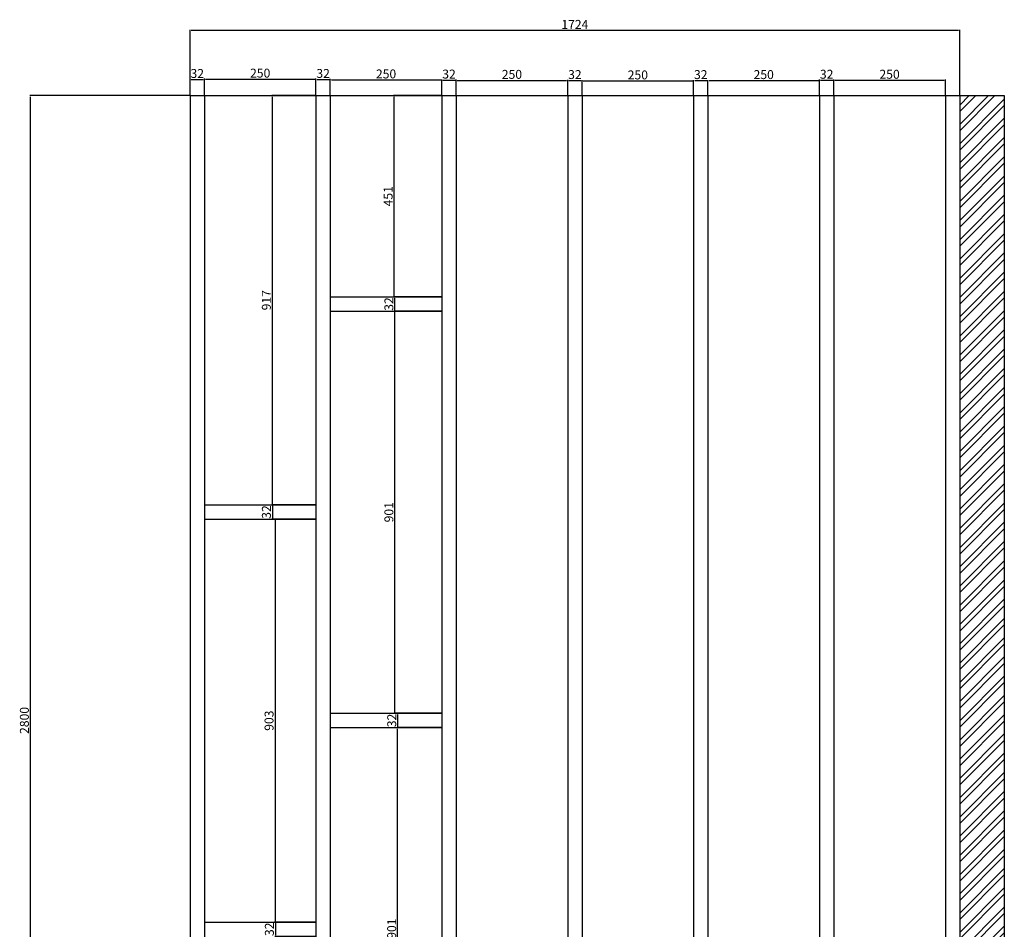
# Model space of a CAD drawing. Units: millimetres. Extents: x 1898 to 8115, y 727 to 4291.
# Tile 2 of 7: x 1898 to 4104, y 2252 to 4291. Entities that reach past the tile are written whole.
import ezdxf

# ---------------------------------------------------------------- set-up
doc = ezdxf.new("R2010")
doc.units = ezdxf.units.MM
for name, color, linetype, lineweight in [('A-ANNO-DIMS', 2, 'Continuous', 18), ('A-DETL', 7, 'Continuous', 25), ('A-DETL-PATT', 8, 'Continuous', 13)]:
    doc.layers.add(name, color=color, linetype=linetype, lineweight=lineweight)
doc.styles.get("Standard").update_dxf_attribs({"font": 'arial.ttf'})
doc.dimstyles.new('ISO-25', dxfattribs={"dimtxt": 20, "dimasz": 2.5, "dimexe": 1.25, "dimexo": 0.625, "dimtad": 1, "dimtxsty": 'Standard', "dimcen": 2.5, "dimadec": 0, "dimazin": 0, "dimtfac": 1, "dimtmove": 0, "dimatfit": 3, "dimfxl": 1, "dimarcsym": 0})

# ---------------------------------------------------------------- blocks, each defined once
blk = doc.blocks.new('*D16')
at = {"layer": 'A-ANNO-DIMS', "color": 0, "lineweight": -2, "transparency": 16777216}
for p, q in [((2279.1, 4120.5), (1920.7, 4120.5)), ((1921.9, 1323), (1921.9, 4118)), ((2279.1, 1320.5), (1920.7, 1320.5))]:
    blk.add_line(p, q, dxfattribs=at)
at = {"layer": 'A-ANNO-DIMS', "color": 0, "transparency": 16777216}
for points in [[(1921.5, 4118), (1922.3, 4118), (1921.9, 4120.5)], [(1921.5, 1323), (1922.3, 1323), (1921.9, 1320.5)]]:
    blk.add_solid(points, dxfattribs=at)
at = {"layer": 'Defpoints', "color": 0, "transparency": 16777216}
for p in [(1921.9, 4120.5), (2279.7, 4120.5), (2279.7, 1320.5)]:
    blk.add_point(p, dxfattribs=at)
at = {"layer": 'A-ANNO-DIMS', "color": 0, "transparency": 16777216, "insert": (1911.1, 2720.5), "char_height": 20, "attachment_point": 5, "rotation": 90}
blk.add_mtext('2800', dxfattribs=at)
blk = doc.blocks.new('*D17')
at = {"layer": 'A-ANNO-DIMS', "color": 0, "lineweight": -2, "transparency": 16777216}
for p, q in [((2279.7, 4121.1), (2279.7, 4268.1)), ((2282.2, 4266.9), (4001.2, 4266.9)), ((4003.7, 4121.1), (4003.7, 4268.1))]:
    blk.add_line(p, q, dxfattribs=at)
at = {"layer": 'A-ANNO-DIMS', "color": 0, "transparency": 16777216}
for points in [[(2282.2, 4267.3), (2282.2, 4266.4), (2279.7, 4266.9)], [(4001.2, 4267.3), (4001.2, 4266.4), (4003.7, 4266.9)]]:
    blk.add_solid(points, dxfattribs=at)
at = {"layer": 'Defpoints', "color": 0, "transparency": 16777216}
for p in [(4003.7, 4266.9), (2279.7, 4120.5), (4003.7, 4120.5)]:
    blk.add_point(p, dxfattribs=at)
at = {"layer": 'A-ANNO-DIMS', "color": 0, "transparency": 16777216, "insert": (3141.7, 4277.5), "char_height": 20, "attachment_point": 5}
blk.add_mtext('1724', dxfattribs=at)
blk = doc.blocks.new('*D18')
at = {"layer": 'A-ANNO-DIMS', "color": 0, "lineweight": -2, "transparency": 16777216}
for p, q in [((2279.7, 4121.1), (2279.7, 4158)), ((2282.2, 4156.8), (2309.2, 4156.8)), ((2311.7, 4121.1), (2311.7, 4158))]:
    blk.add_line(p, q, dxfattribs=at)
at = {"layer": 'A-ANNO-DIMS', "color": 0, "transparency": 16777216}
for points in [[(2282.2, 4157.2), (2282.2, 4156.4), (2279.7, 4156.8)], [(2309.2, 4157.2), (2309.2, 4156.4), (2311.7, 4156.8)]]:
    blk.add_solid(points, dxfattribs=at)
at = {"layer": 'Defpoints', "color": 0, "transparency": 16777216}
for p in [(2311.7, 4156.8), (2279.7, 4120.5), (2311.7, 4120.5)]:
    blk.add_point(p, dxfattribs=at)
at = {"layer": 'A-ANNO-DIMS', "color": 0, "transparency": 16777216, "insert": (2295.7, 4167.6), "char_height": 20, "attachment_point": 5}
blk.add_mtext('32', dxfattribs=at)
blk = doc.blocks.new('*D19')
at = {"layer": 'A-ANNO-DIMS', "color": 0, "lineweight": -2, "transparency": 16777216}
for p, q in [((2311.7, 4121.1), (2311.7, 4158.7)), ((2314.2, 4157.5), (2559.2, 4157.5)), ((2561.7, 4121.1), (2561.7, 4158.7))]:
    blk.add_line(p, q, dxfattribs=at)
at = {"layer": 'A-ANNO-DIMS', "color": 0, "transparency": 16777216}
for points in [[(2314.2, 4157.9), (2314.2, 4157), (2311.7, 4157.5)], [(2559.2, 4157.9), (2559.2, 4157), (2561.7, 4157.5)]]:
    blk.add_solid(points, dxfattribs=at)
at = {"layer": 'Defpoints', "color": 0, "transparency": 16777216}
for p in [(2561.7, 4157.5), (2311.7, 4120.5), (2561.7, 4120.5)]:
    blk.add_point(p, dxfattribs=at)
at = {"layer": 'A-ANNO-DIMS', "color": 0, "transparency": 16777216, "insert": (2436.7, 4168.3), "char_height": 20, "attachment_point": 5}
blk.add_mtext('250', dxfattribs=at)
blk = doc.blocks.new('*D20')
at = {"layer": 'A-ANNO-DIMS', "color": 0, "lineweight": -2, "transparency": 16777216}
for p, q in [((2561.7, 4121.1), (2561.7, 4158)), ((2564.2, 4156.8), (2591.2, 4156.8)), ((2593.7, 4121.1), (2593.7, 4158))]:
    blk.add_line(p, q, dxfattribs=at)
at = {"layer": 'A-ANNO-DIMS', "color": 0, "transparency": 16777216}
for points in [[(2564.2, 4157.2), (2564.2, 4156.4), (2561.7, 4156.8)], [(2591.2, 4157.2), (2591.2, 4156.4), (2593.7, 4156.8)]]:
    blk.add_solid(points, dxfattribs=at)
at = {"layer": 'Defpoints', "color": 0, "transparency": 16777216}
for p in [(2593.7, 4156.8), (2561.7, 4120.5), (2593.7, 4120.5)]:
    blk.add_point(p, dxfattribs=at)
at = {"layer": 'A-ANNO-DIMS', "color": 0, "transparency": 16777216, "insert": (2577.7, 4167.6), "char_height": 20, "attachment_point": 5}
blk.add_mtext('32', dxfattribs=at)
blk = doc.blocks.new('*D21')
at = {"layer": 'A-ANNO-DIMS', "color": 0, "lineweight": -2, "transparency": 16777216}
for p, q in [((2593.7, 4121.1), (2593.7, 4156.9)), ((2596.2, 4155.7), (2841.2, 4155.7)), ((2843.7, 4121.1), (2843.7, 4156.9))]:
    blk.add_line(p, q, dxfattribs=at)
at = {"layer": 'A-ANNO-DIMS', "color": 0, "transparency": 16777216}
for points in [[(2596.2, 4156.1), (2596.2, 4155.3), (2593.7, 4155.7)], [(2841.2, 4156.1), (2841.2, 4155.3), (2843.7, 4155.7)]]:
    blk.add_solid(points, dxfattribs=at)
at = {"layer": 'Defpoints', "color": 0, "transparency": 16777216}
for p in [(2843.7, 4155.7), (2593.7, 4120.5), (2843.7, 4120.5)]:
    blk.add_point(p, dxfattribs=at)
at = {"layer": 'A-ANNO-DIMS', "color": 0, "transparency": 16777216, "insert": (2718.7, 4166.5), "char_height": 20, "attachment_point": 5}
blk.add_mtext('250', dxfattribs=at)
blk = doc.blocks.new('*D22')
at = {"layer": 'A-ANNO-DIMS', "color": 0, "lineweight": -2, "transparency": 16777216}
for p, q in [((2843.7, 4121.1), (2843.7, 4156.6)), ((2846.2, 4155.3), (2873.2, 4155.3)), ((2875.7, 4121.1), (2875.7, 4156.6))]:
    blk.add_line(p, q, dxfattribs=at)
at = {"layer": 'A-ANNO-DIMS', "color": 0, "transparency": 16777216}
for points in [[(2846.2, 4155.8), (2846.2, 4154.9), (2843.7, 4155.3)], [(2873.2, 4155.8), (2873.2, 4154.9), (2875.7, 4155.3)]]:
    blk.add_solid(points, dxfattribs=at)
at = {"layer": 'Defpoints', "color": 0, "transparency": 16777216}
for p in [(2875.7, 4155.3), (2843.7, 4120.5), (2875.7, 4120.5)]:
    blk.add_point(p, dxfattribs=at)
at = {"layer": 'A-ANNO-DIMS', "color": 0, "transparency": 16777216, "insert": (2859.7, 4166.2), "char_height": 20, "attachment_point": 5}
blk.add_mtext('32', dxfattribs=at)
blk = doc.blocks.new('*D23')
at = {"layer": 'A-ANNO-DIMS', "color": 0, "lineweight": -2, "transparency": 16777216}
for p, q in [((2875.7, 4121.1), (2875.7, 4155.9)), ((2878.2, 4154.6), (3123.2, 4154.6)), ((3125.7, 4121.1), (3125.7, 4155.9))]:
    blk.add_line(p, q, dxfattribs=at)
at = {"layer": 'A-ANNO-DIMS', "color": 0, "transparency": 16777216}
for points in [[(2878.2, 4155.1), (2878.2, 4154.2), (2875.7, 4154.6)], [(3123.2, 4155.1), (3123.2, 4154.2), (3125.7, 4154.6)]]:
    blk.add_solid(points, dxfattribs=at)
at = {"layer": 'Defpoints', "color": 0, "transparency": 16777216}
for p in [(3125.7, 4154.6), (2875.7, 4120.5), (3125.7, 4120.5)]:
    blk.add_point(p, dxfattribs=at)
at = {"layer": 'A-ANNO-DIMS', "color": 0, "transparency": 16777216, "insert": (3000.7, 4165.5), "char_height": 20, "attachment_point": 5}
blk.add_mtext('250', dxfattribs=at)
blk = doc.blocks.new('*D24')
at = {"layer": 'A-ANNO-DIMS', "color": 0, "lineweight": -2, "transparency": 16777216}
for p, q in [((3125.7, 4121.1), (3125.7, 4155.5)), ((3128.2, 4154.2), (3155.2, 4154.2)), ((3157.7, 4121.1), (3157.7, 4155.5))]:
    blk.add_line(p, q, dxfattribs=at)
at = {"layer": 'A-ANNO-DIMS', "color": 0, "transparency": 16777216}
for points in [[(3128.2, 4154.6), (3128.2, 4153.8), (3125.7, 4154.2)], [(3155.2, 4154.6), (3155.2, 4153.8), (3157.7, 4154.2)]]:
    blk.add_solid(points, dxfattribs=at)
at = {"layer": 'Defpoints', "color": 0, "transparency": 16777216}
for p in [(3157.7, 4154.2), (3125.7, 4120.5), (3157.7, 4120.5)]:
    blk.add_point(p, dxfattribs=at)
at = {"layer": 'A-ANNO-DIMS', "color": 0, "transparency": 16777216, "insert": (3141.7, 4165.1), "char_height": 20, "attachment_point": 5}
blk.add_mtext('32', dxfattribs=at)
blk = doc.blocks.new('*D25')
at = {"layer": 'A-ANNO-DIMS', "color": 0, "lineweight": -2, "transparency": 16777216}
for p, q in [((3157.7, 4121.1), (3157.7, 4154.7)), ((3160.2, 4153.4), (3405.2, 4153.4)), ((3407.7, 4121.1), (3407.7, 4154.7))]:
    blk.add_line(p, q, dxfattribs=at)
at = {"layer": 'A-ANNO-DIMS', "color": 0, "transparency": 16777216}
for points in [[(3160.2, 4153.8), (3160.2, 4153), (3157.7, 4153.4)], [(3405.2, 4153.8), (3405.2, 4153), (3407.7, 4153.4)]]:
    blk.add_solid(points, dxfattribs=at)
at = {"layer": 'Defpoints', "color": 0, "transparency": 16777216}
for p in [(3407.7, 4153.4), (3157.7, 4120.5), (3407.7, 4120.5)]:
    blk.add_point(p, dxfattribs=at)
at = {"layer": 'A-ANNO-DIMS', "color": 0, "transparency": 16777216, "insert": (3282.7, 4164.3), "char_height": 20, "attachment_point": 5}
blk.add_mtext('250', dxfattribs=at)
blk = doc.blocks.new('*D26')
at = {"layer": 'A-ANNO-DIMS', "color": 0, "lineweight": -2, "transparency": 16777216}
for p, q in [((3439.7, 4121.1), (3439.7, 4155.4)), ((3442.2, 4154.1), (3687.2, 4154.1)), ((3689.7, 4121.1), (3689.7, 4155.4))]:
    blk.add_line(p, q, dxfattribs=at)
at = {"layer": 'A-ANNO-DIMS', "color": 0, "transparency": 16777216}
for points in [[(3442.2, 4154.5), (3442.2, 4153.7), (3439.7, 4154.1)], [(3687.2, 4154.5), (3687.2, 4153.7), (3689.7, 4154.1)]]:
    blk.add_solid(points, dxfattribs=at)
at = {"layer": 'Defpoints', "color": 0, "transparency": 16777216}
for p in [(3689.7, 4154.1), (3439.7, 4120.5), (3689.7, 4120.5)]:
    blk.add_point(p, dxfattribs=at)
at = {"layer": 'A-ANNO-DIMS', "color": 0, "transparency": 16777216, "insert": (3564.7, 4165), "char_height": 20, "attachment_point": 5}
blk.add_mtext('250', dxfattribs=at)
blk = doc.blocks.new('*D27')
at = {"layer": 'A-ANNO-DIMS', "color": 0, "lineweight": -2, "transparency": 16777216}
for p, q in [((3721.7, 4121.1), (3721.7, 4156.3)), ((3724.2, 4155), (3969.2, 4155)), ((3971.7, 4121.1), (3971.7, 4156.3))]:
    blk.add_line(p, q, dxfattribs=at)
at = {"layer": 'A-ANNO-DIMS', "color": 0, "transparency": 16777216}
for points in [[(3724.2, 4155.4), (3724.2, 4154.6), (3721.7, 4155)], [(3969.2, 4155.4), (3969.2, 4154.6), (3971.7, 4155)]]:
    blk.add_solid(points, dxfattribs=at)
at = {"layer": 'Defpoints', "color": 0, "transparency": 16777216}
for p in [(3971.7, 4155), (3721.7, 4120.5), (3971.7, 4120.5)]:
    blk.add_point(p, dxfattribs=at)
at = {"layer": 'A-ANNO-DIMS', "color": 0, "transparency": 16777216, "insert": (3846.7, 4165.8), "char_height": 20, "attachment_point": 5}
blk.add_mtext('250', dxfattribs=at)
blk = doc.blocks.new('*D28')
at = {"layer": 'A-ANNO-DIMS', "color": 0, "lineweight": -2, "transparency": 16777216}
for p, q in [((3689.7, 4121.1), (3689.7, 4156.3)), ((3692.2, 4155), (3719.2, 4155)), ((3721.7, 4121.1), (3721.7, 4156.3))]:
    blk.add_line(p, q, dxfattribs=at)
at = {"layer": 'A-ANNO-DIMS', "color": 0, "transparency": 16777216}
for points in [[(3692.2, 4155.4), (3692.2, 4154.6), (3689.7, 4155)], [(3719.2, 4155.4), (3719.2, 4154.6), (3721.7, 4155)]]:
    blk.add_solid(points, dxfattribs=at)
at = {"layer": 'Defpoints', "color": 0, "transparency": 16777216}
for p in [(3721.7, 4155), (3689.7, 4120.5), (3721.7, 4120.5)]:
    blk.add_point(p, dxfattribs=at)
at = {"layer": 'A-ANNO-DIMS', "color": 0, "transparency": 16777216, "insert": (3705.7, 4165.8), "char_height": 20, "attachment_point": 5}
blk.add_mtext('32', dxfattribs=at)
blk = doc.blocks.new('*D29')
at = {"layer": 'A-ANNO-DIMS', "color": 0, "lineweight": -2, "transparency": 16777216}
for p, q in [((3407.7, 4121.1), (3407.7, 4155.4)), ((3410.2, 4154.1), (3437.2, 4154.1)), ((3439.7, 4121.1), (3439.7, 4155.4))]:
    blk.add_line(p, q, dxfattribs=at)
at = {"layer": 'A-ANNO-DIMS', "color": 0, "transparency": 16777216}
for points in [[(3410.2, 4154.5), (3410.2, 4153.7), (3407.7, 4154.1)], [(3437.2, 4154.5), (3437.2, 4153.7), (3439.7, 4154.1)]]:
    blk.add_solid(points, dxfattribs=at)
at = {"layer": 'Defpoints', "color": 0, "transparency": 16777216}
for p in [(3439.7, 4154.1), (3407.7, 4120.5), (3439.7, 4120.5)]:
    blk.add_point(p, dxfattribs=at)
at = {"layer": 'A-ANNO-DIMS', "color": 0, "transparency": 16777216, "insert": (3423.7, 4165), "char_height": 20, "attachment_point": 5}
blk.add_mtext('32', dxfattribs=at)
blk = doc.blocks.new('*D30')
at = {"layer": 'A-ANNO-DIMS', "color": 0, "lineweight": -2, "transparency": 16777216}
for p, q in [((2561.1, 4120.5), (2462.7, 4120.5)), ((2463.9, 4118), (2463.9, 3206)), ((2561.1, 3203.5), (2462.7, 3203.5))]:
    blk.add_line(p, q, dxfattribs=at)
at = {"layer": 'A-ANNO-DIMS', "color": 0, "transparency": 16777216}
for points in [[(2463.5, 4118), (2464.4, 4118), (2463.9, 4120.5)], [(2463.5, 3206), (2464.4, 3206), (2463.9, 3203.5)]]:
    blk.add_solid(points, dxfattribs=at)
at = {"layer": 'Defpoints', "color": 0, "transparency": 16777216}
for p in [(2561.7, 4120.5), (2463.9, 3203.5), (2561.7, 3203.5)]:
    blk.add_point(p, dxfattribs=at)
at = {"layer": 'A-ANNO-DIMS', "color": 0, "transparency": 16777216, "insert": (2453.1, 3662), "char_height": 20, "attachment_point": 5, "rotation": 90}
blk.add_mtext('917', dxfattribs=at)
blk = doc.blocks.new('*D31')
at = {"layer": 'A-ANNO-DIMS', "color": 0, "lineweight": -2, "transparency": 16777216}
for p, q in [((2561.1, 3203.5), (2462.8, 3203.5)), ((2464, 3201), (2464, 3174)), ((2561.1, 3171.5), (2462.8, 3171.5))]:
    blk.add_line(p, q, dxfattribs=at)
at = {"layer": 'A-ANNO-DIMS', "color": 0, "transparency": 16777216}
for points in [[(2463.6, 3201), (2464.4, 3201), (2464, 3203.5)], [(2463.6, 3174), (2464.4, 3174), (2464, 3171.5)]]:
    blk.add_solid(points, dxfattribs=at)
at = {"layer": 'Defpoints', "color": 0, "transparency": 16777216}
for p in [(2561.7, 3203.5), (2464, 3171.5), (2561.7, 3171.5)]:
    blk.add_point(p, dxfattribs=at)
at = {"layer": 'A-ANNO-DIMS', "color": 0, "transparency": 16777216, "insert": (2453.2, 3187.5), "char_height": 20, "attachment_point": 5, "rotation": 90}
blk.add_mtext('32', dxfattribs=at)
blk = doc.blocks.new('*D32')
at = {"layer": 'A-ANNO-DIMS', "color": 0, "lineweight": -2, "transparency": 16777216}
for p, q in [((2561.1, 3171.5), (2468.8, 3171.5)), ((2470, 3169), (2470, 2271)), ((2561.1, 2268.5), (2468.8, 2268.5))]:
    blk.add_line(p, q, dxfattribs=at)
at = {"layer": 'A-ANNO-DIMS', "color": 0, "transparency": 16777216}
for points in [[(2469.6, 3169), (2470.4, 3169), (2470, 3171.5)], [(2469.6, 2271), (2470.4, 2271), (2470, 2268.5)]]:
    blk.add_solid(points, dxfattribs=at)
at = {"layer": 'Defpoints', "color": 0, "transparency": 16777216}
for p in [(2561.7, 3171.5), (2470, 2268.5), (2561.7, 2268.5)]:
    blk.add_point(p, dxfattribs=at)
at = {"layer": 'A-ANNO-DIMS', "color": 0, "transparency": 16777216, "insert": (2459.2, 2720), "char_height": 20, "attachment_point": 5, "rotation": 90}
blk.add_mtext('903', dxfattribs=at)
blk = doc.blocks.new('*D33')
at = {"layer": 'A-ANNO-DIMS', "color": 0, "lineweight": -2, "transparency": 16777216}
for p, q in [((2561.1, 2268.5), (2469.5, 2268.5)), ((2470.7, 2266), (2470.7, 2239)), ((2561.1, 2236.5), (2469.5, 2236.5))]:
    blk.add_line(p, q, dxfattribs=at)
at = {"layer": 'A-ANNO-DIMS', "color": 0, "transparency": 16777216}
for points in [[(2470.3, 2266), (2471.2, 2266), (2470.7, 2268.5)], [(2470.3, 2239), (2471.2, 2239), (2470.7, 2236.5)]]:
    blk.add_solid(points, dxfattribs=at)
at = {"layer": 'Defpoints', "color": 0, "transparency": 16777216}
for p in [(2561.7, 2268.5), (2470.7, 2236.5), (2561.7, 2236.5)]:
    blk.add_point(p, dxfattribs=at)
at = {"layer": 'A-ANNO-DIMS', "color": 0, "transparency": 16777216, "insert": (2459.9, 2252.5), "char_height": 20, "attachment_point": 5, "rotation": 90}
blk.add_mtext('32', dxfattribs=at)
blk = doc.blocks.new('*D37')
at = {"layer": 'A-ANNO-DIMS', "color": 0, "lineweight": -2, "transparency": 16777216}
for p, q in [((2843.1, 2704.5), (2743.4, 2704.5)), ((2744.7, 1806), (2744.7, 2702)), ((2843.1, 1803.5), (2743.4, 1803.5))]:
    blk.add_line(p, q, dxfattribs=at)
at = {"layer": 'A-ANNO-DIMS', "color": 0, "transparency": 16777216}
for points in [[(2744.3, 2702), (2745.1, 2702), (2744.7, 2704.5)], [(2744.3, 1806), (2745.1, 1806), (2744.7, 1803.5)]]:
    blk.add_solid(points, dxfattribs=at)
at = {"layer": 'Defpoints', "color": 0, "transparency": 16777216}
for p in [(2744.7, 2704.5), (2843.7, 2704.5), (2843.7, 1803.5)]:
    blk.add_point(p, dxfattribs=at)
at = {"layer": 'A-ANNO-DIMS', "color": 0, "transparency": 16777216, "insert": (2733.8, 2254), "char_height": 20, "attachment_point": 5, "rotation": 90}
blk.add_mtext('901', dxfattribs=at)
blk = doc.blocks.new('*D38')
at = {"layer": 'A-ANNO-DIMS', "color": 0, "lineweight": -2, "transparency": 16777216}
for p, q in [((2843.1, 2736.5), (2743.6, 2736.5)), ((2744.9, 2707), (2744.9, 2734)), ((2843.1, 2704.5), (2743.6, 2704.5))]:
    blk.add_line(p, q, dxfattribs=at)
at = {"layer": 'A-ANNO-DIMS', "color": 0, "transparency": 16777216}
for points in [[(2744.5, 2734), (2745.3, 2734), (2744.9, 2736.5)], [(2744.5, 2707), (2745.3, 2707), (2744.9, 2704.5)]]:
    blk.add_solid(points, dxfattribs=at)
at = {"layer": 'Defpoints', "color": 0, "transparency": 16777216}
for p in [(2744.9, 2736.5), (2843.7, 2736.5), (2843.7, 2704.5)]:
    blk.add_point(p, dxfattribs=at)
at = {"layer": 'A-ANNO-DIMS', "color": 0, "transparency": 16777216, "insert": (2734, 2720.5), "char_height": 20, "attachment_point": 5, "rotation": 90}
blk.add_mtext('32', dxfattribs=at)
blk = doc.blocks.new('*D39')
at = {"layer": 'A-ANNO-DIMS', "color": 0, "lineweight": -2, "transparency": 16777216}
for p, q in [((2843.1, 3637.5), (2737.2, 3637.5)), ((2738.5, 2739), (2738.5, 3635)), ((2843.1, 2736.5), (2737.2, 2736.5))]:
    blk.add_line(p, q, dxfattribs=at)
at = {"layer": 'A-ANNO-DIMS', "color": 0, "transparency": 16777216}
for points in [[(2738.1, 3635), (2738.9, 3635), (2738.5, 3637.5)], [(2738.1, 2739), (2738.9, 2739), (2738.5, 2736.5)]]:
    blk.add_solid(points, dxfattribs=at)
at = {"layer": 'Defpoints', "color": 0, "transparency": 16777216}
for p in [(2738.5, 3637.5), (2843.7, 3637.5), (2843.7, 2736.5)]:
    blk.add_point(p, dxfattribs=at)
at = {"layer": 'A-ANNO-DIMS', "color": 0, "transparency": 16777216, "insert": (2727.6, 3187), "char_height": 20, "attachment_point": 5, "rotation": 90}
blk.add_mtext('901', dxfattribs=at)
blk = doc.blocks.new('*D40')
at = {"layer": 'A-ANNO-DIMS', "color": 0, "lineweight": -2, "transparency": 16777216}
for p, q in [((2843.1, 3669.5), (2737.2, 3669.5)), ((2738.5, 3640), (2738.5, 3667)), ((2843.1, 3637.5), (2737.2, 3637.5))]:
    blk.add_line(p, q, dxfattribs=at)
at = {"layer": 'A-ANNO-DIMS', "color": 0, "transparency": 16777216}
for points in [[(2738.1, 3667), (2738.9, 3667), (2738.5, 3669.5)], [(2738.1, 3640), (2738.9, 3640), (2738.5, 3637.5)]]:
    blk.add_solid(points, dxfattribs=at)
at = {"layer": 'Defpoints', "color": 0, "transparency": 16777216}
for p in [(2738.5, 3669.5), (2843.7, 3669.5), (2843.7, 3637.5)]:
    blk.add_point(p, dxfattribs=at)
at = {"layer": 'A-ANNO-DIMS', "color": 0, "transparency": 16777216, "insert": (2727.6, 3653.5), "char_height": 20, "attachment_point": 5, "rotation": 90}
blk.add_mtext('32', dxfattribs=at)
blk = doc.blocks.new('*D41')
at = {"layer": 'A-ANNO-DIMS', "color": 0, "lineweight": -2, "transparency": 16777216}
for p, q in [((2843.1, 4120.5), (2735.5, 4120.5)), ((2736.8, 3672), (2736.8, 4118)), ((2843.1, 3669.5), (2735.5, 3669.5))]:
    blk.add_line(p, q, dxfattribs=at)
at = {"layer": 'A-ANNO-DIMS', "color": 0, "transparency": 16777216}
for points in [[(2736.4, 4118), (2737.2, 4118), (2736.8, 4120.5)], [(2736.4, 3672), (2737.2, 3672), (2736.8, 3669.5)]]:
    blk.add_solid(points, dxfattribs=at)
at = {"layer": 'Defpoints', "color": 0, "transparency": 16777216}
for p in [(2736.8, 4120.5), (2843.7, 4120.5), (2843.7, 3669.5)]:
    blk.add_point(p, dxfattribs=at)
at = {"layer": 'A-ANNO-DIMS', "color": 0, "transparency": 16777216, "insert": (2725.9, 3895), "char_height": 20, "attachment_point": 5, "rotation": 90}
blk.add_mtext('451', dxfattribs=at)

msp = doc.modelspace()

# ---------------------------------------------------------------- hatches: boundary and pattern name
at = {"layer": 'A-DETL-PATT'}
h = msp.add_hatch(dxfattribs=at)
h.set_pattern_fill('ANSI32', color=256, scale=3.2)
h.set_pattern_definition([(45, (132, 2037.696), (-21.55261, 21.55261), []), (45, (146.368, 2037.696), (-21.55261, 21.55261), [])])
h.paths.add_polyline_path([(4003.701, 1320.491), (4103.701, 1320.491), (4103.701, 4120.491), (4003.701, 4120.491)])

# ---------------------------------------------------------------- linework, layer by layer
at = {"layer": 'A-DETL'}
for p, q in [((2279.701, 4120.491), (2311.701, 4120.491)), ((2279.701, 4120.491), (2279.701, 3976.996)), ((2279.701, 4120.491), (2279.701, 1320.491)), ((2311.701, 4120.491), (2311.701, 4071.26)), ((2311.701, 4120.491), (2561.701, 4120.491)), ((2311.701, 4120.491), (2311.701, 3203.491)), ((2561.701, 4120.491), (2561.701, 4071.663)), ((2561.701, 4120.491), (2593.701, 4120.491)), ((2593.701, 4120.491), (2593.701, 4077.96)), ((2593.701, 4120.491), (2843.701, 4120.491)), ((2593.701, 4120.491), (2593.701, 3669.491)), ((2843.701, 4120.491), (2843.701, 4101.573)), ((2843.701, 4120.491), (2875.701, 4120.491)), ((2843.701, 4120.491), (2843.701, 1320.491)), ((2875.701, 4120.491), (2875.701, 4108.716)), ((2875.701, 4120.491), (3125.701, 4120.491)), ((2875.701, 4120.491), (2875.701, 1320.491)), ((2875.701, 4120.491), (2875.701, 3669.491)), ((3125.701, 4120.491), (3125.701, 4087.257)), ((3125.701, 4120.491), (3157.701, 4120.491)), ((3157.701, 4120.491), (3157.701, 4070.861)), ((3157.701, 4120.491), (3407.701, 4120.491)), ((3407.701, 4120.491), (3407.701, 4092.434)), ((3407.701, 4120.491), (3439.701, 4120.491)), ((3407.701, 4106.462), (3407.701, 1320.491)), ((3439.701, 4120.491), (3439.701, 4083.546)), ((3439.701, 4120.491), (3689.701, 4120.491)), ((3689.701, 4120.491), (3689.701, 4096.592)), ((3689.701, 4120.491), (3721.701, 4120.491)), ((3721.701, 4120.491), (3721.701, 4089.634)), ((3721.701, 4120.491), (3971.701, 4120.491)), ((3971.701, 4120.491), (3971.701, 4105.584)), ((3971.701, 4120.491), (4003.701, 4120.491)), ((3971.701, 4120.491), (3971.701, 1320.491)), ((4003.701, 4120.491), (4003.701, 1320.491)), ((4003.701, 4120.491), (4103.701, 4120.491)), ((4103.701, 4120.491), (4103.701, 1320.491)), ((3125.701, 4087.257), (3125.701, 1320.491)), ((3439.701, 4083.546), (3439.701, 1320.491)), ((3689.701, 4096.592), (3689.701, 1320.491)), ((3721.701, 4089.634), (3721.701, 1320.491)), ((2311.701, 4071.26), (2311.701, 1320.491)), ((2561.701, 4071.663), (2561.701, 1320.491)), ((2593.701, 4077.96), (2593.701, 1320.491)), ((3157.701, 4070.861), (3157.701, 1320.491)), ((2593.701, 3669.491), (2843.701, 3669.491)), ((2593.701, 3637.491), (2843.701, 3637.491)), ((2311.701, 3203.491), (2561.701, 3203.491)), ((2311.701, 3171.491), (2561.701, 3171.491)), ((2311.701, 3171.491), (2311.701, 2268.491)), ((2593.701, 2736.491), (2843.701, 2736.491)), ((2593.701, 2704.491), (2843.701, 2704.491)), ((2311.701, 2268.491), (2561.701, 2268.491))]:
    msp.add_line(p, q, dxfattribs=at)

# ---------------------------------------------------------------- dimensions: what is measured, and where the dimension line sits
at = {"layer": 'A-ANNO-DIMS'}
for base, p1, p2, picture, middle in [((4003.701, 4266.863), (2279.701, 4120.491), (4003.701, 4120.491), '*D17', (3141.701, 4277.528)), ((2311.701, 4156.778), (2279.701, 4120.491), (2311.701, 4120.491), '*D18', (2295.701, 4167.621)), ((2561.701, 4157.457), (2311.701, 4120.491), (2561.701, 4120.491), '*D19', (2436.701, 4168.294)), ((2593.701, 4156.778), (2561.701, 4120.491), (2593.701, 4120.491), '*D20', (2577.701, 4167.621)), ((2843.701, 4155.673), (2593.701, 4120.491), (2843.701, 4120.491), '*D21', (2718.701, 4166.509)), ((2875.701, 4155.346), (2843.701, 4120.491), (2875.701, 4120.491), '*D22', (2859.701, 4166.189)), ((3125.701, 4154.649), (2875.701, 4120.491), (3125.701, 4120.491), '*D23', (3000.701, 4165.486)), ((3157.701, 4154.211), (3125.701, 4120.491), (3157.701, 4120.491), '*D24', (3141.701, 4165.054)), ((3407.701, 4153.414), (3157.701, 4120.491), (3407.701, 4120.491), '*D25', (3282.701, 4164.251)), ((3439.701, 4154.118), (3407.701, 4120.491), (3439.701, 4120.491), '*D29', (3423.701, 4164.961)), ((3689.701, 4154.118), (3439.701, 4120.491), (3689.701, 4120.491), '*D26', (3564.701, 4164.955)), ((3721.701, 4155), (3689.701, 4120.491), (3721.701, 4120.491), '*D28', (3705.701, 4165.844)), ((3971.701, 4155), (3721.701, 4120.491), (3971.701, 4120.491), '*D27', (3846.701, 4165.837))]:
    dim = msp.add_linear_dim(base=base, p1=p1, p2=p2, dimstyle='ISO-25', override={"dimclrd": 0, "dimclre": 0, "dimclrt": 0}, dxfattribs=at)
    dim.commit()
    dim.dimension.update_dxf_attribs({"geometry": picture, "text_midpoint": middle})
for base, p1, p2, picture, middle in [((1921.926, 4120.491), (2279.701, 1320.491), (2279.701, 4120.491), '*D16', (1911.089, 2720.491)), ((2463.94, 3203.491), (2561.701, 4120.491), (2561.701, 3203.491), '*D30', (2453.104, 3661.991)), ((2736.777, 4120.491), (2843.701, 3669.491), (2843.701, 4120.491), '*D41', (2725.941, 3894.991)), ((2738.468, 3669.491), (2843.701, 3637.491), (2843.701, 3669.491), '*D40', (2727.625, 3653.491)), ((2738.476, 3637.491), (2843.701, 2736.491), (2843.701, 3637.491), '*D39', (2727.639, 3186.991)), ((2464.023, 3171.491), (2561.701, 3203.491), (2561.701, 3171.491), '*D31', (2453.18, 3187.491)), ((2470.009, 2268.491), (2561.701, 3171.491), (2561.701, 2268.491), '*D32', (2459.166, 2719.991)), ((2744.871, 2736.491), (2843.701, 2704.491), (2843.701, 2736.491), '*D38', (2734.028, 2720.491)), ((2744.671, 2704.491), (2843.701, 1803.491), (2843.701, 2704.491), '*D37', (2733.834, 2253.991)), ((2470.75, 2236.491), (2561.701, 2268.491), (2561.701, 2236.491), '*D33', (2459.906, 2252.491))]:
    dim = msp.add_linear_dim(base=base, p1=p1, p2=p2, angle=90, dimstyle='ISO-25', override={"dimclrd": 0, "dimclre": 0, "dimclrt": 0}, dxfattribs=at)
    dim.commit()
    dim.dimension.update_dxf_attribs({"geometry": picture, "text_midpoint": middle})

doc.saveas('drawing.dxf')
